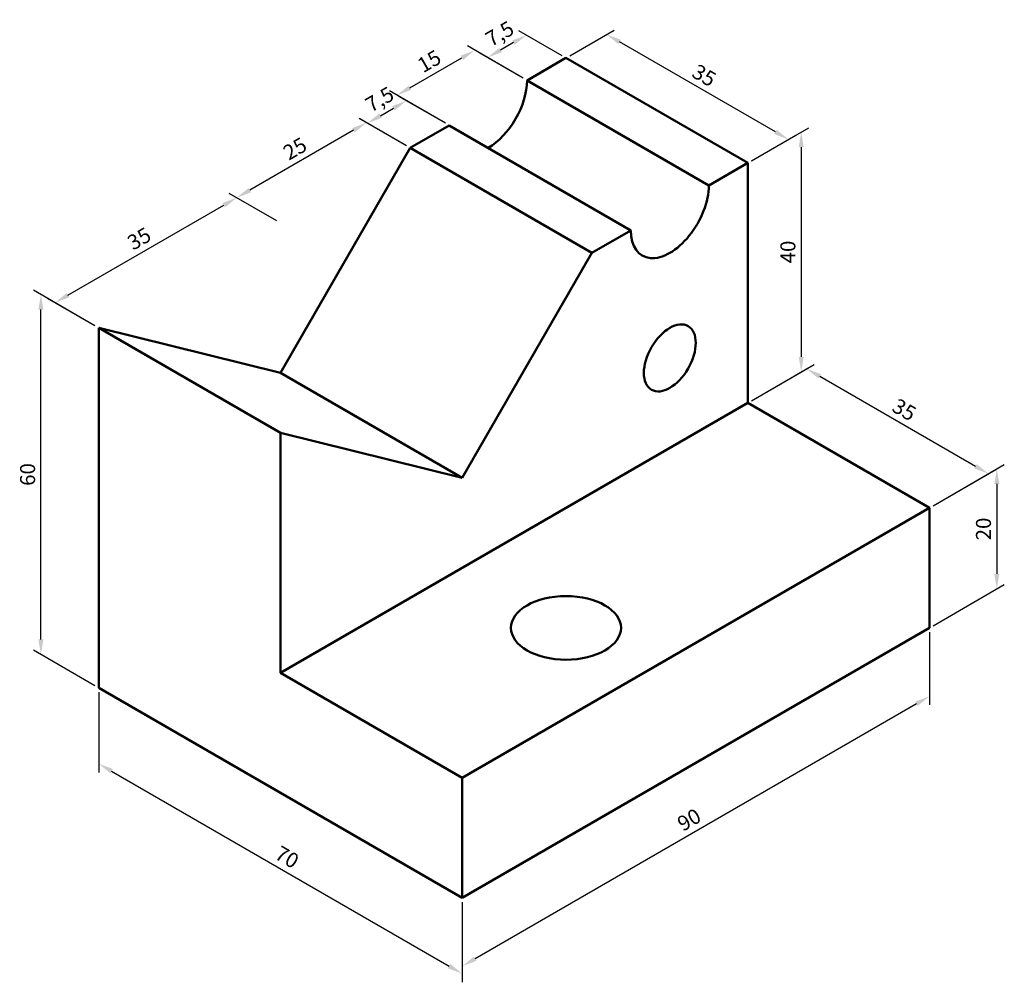
# Model space of a CAD drawing. Units: millimetres. Extents: x 1933 to 2097, y 2342 to 2503.
import ezdxf

# ---------------------------------------------------------------- set-up
doc = ezdxf.new("R2010")
doc.units = ezdxf.units.MM
doc.layers.add('M-DIMS', color=2, linetype='Continuous', lineweight=25)
doc.layers.add('M-OUTL', color=7, linetype='Continuous', lineweight=50)
doc.styles.get("Standard").update_dxf_attribs({"font": 'arial.ttf'})
doc.dimstyles.new('ISO-25', dxfattribs={"dimtxt": 2.5, "dimasz": 2.5, "dimexe": 1.25, "dimexo": 0.625, "dimtad": 1, "dimtxsty": 'Standard', "dimcen": 2.5, "dimadec": 0, "dimazin": 0, "dimtfac": 1, "dimtmove": 0, "dimatfit": 3, "dimfxl": 1, "dimarcsym": 0})

# ---------------------------------------------------------------- blocks, each defined once
blk = doc.blocks.new('*D1')
at = {"layer": 'Defpoints', "color": 0, "transparency": 16777216}
for p in [(2084.43, 2401.38), (2006.49, 2356.38), (2006.49, 2344.97)]:
    blk.add_point(p, dxfattribs=at)
at = {"layer": 'M-DIMS', "color": 0, "lineweight": -2, "transparency": 16777216}
for p, q in [((2084.43, 2400.65), (2084.43, 2388.53)), ((2082.27, 2388.72), (2008.66, 2346.22)), ((2006.49, 2355.65), (2006.49, 2343.53))]:
    blk.add_line(p, q, dxfattribs=at)
at = {"layer": 'M-DIMS', "color": 0, "transparency": 16777216}
for points in [[(2082.06, 2389.08), (2082.48, 2388.36), (2084.43, 2389.97)], [(2008.45, 2346.58), (2008.86, 2345.86), (2006.49, 2344.97)]]:
    blk.add_solid(points, dxfattribs=at)
at = {"layer": 'M-DIMS', "color": 0, "transparency": 16777216, "insert": (2044.51, 2369.12), "char_height": 2.5, "attachment_point": 5, "rotation": 30}
blk.add_mtext('90', dxfattribs=at)
blk = doc.blocks.new('*D2')
at = {"layer": 'Defpoints', "color": 0, "transparency": 16777216}
for p in [(2084.43, 2421.38), (2095.67, 2407.86), (2084.43, 2401.38)]:
    blk.add_point(p, dxfattribs=at)
at = {"layer": 'M-DIMS', "color": 0, "lineweight": -2, "transparency": 16777216}
for p, q in [((2085.06, 2421.74), (2096.92, 2428.59)), ((2095.67, 2425.36), (2095.67, 2410.36)), ((2085.06, 2401.74), (2096.92, 2408.59))]:
    blk.add_line(p, q, dxfattribs=at)
at = {"layer": 'M-DIMS', "color": 0, "transparency": 16777216}
for points in [[(2095.26, 2425.36), (2096.09, 2425.36), (2095.67, 2427.86)], [(2095.26, 2410.36), (2096.09, 2410.36), (2095.67, 2407.86)]]:
    blk.add_solid(points, dxfattribs=at)
at = {"layer": 'M-DIMS', "color": 0, "transparency": 16777216, "insert": (2093.77, 2417.86), "char_height": 2.5, "attachment_point": 5, "rotation": 90}
blk.add_mtext('20', dxfattribs=at)
blk = doc.blocks.new('*D3')
at = {"layer": 'Defpoints', "color": 0, "transparency": 16777216}
for p in [(2054.12, 2438.88), (2094.28, 2427.06), (2084.43, 2421.38)]:
    blk.add_point(p, dxfattribs=at)
at = {"layer": 'M-DIMS', "color": 0, "lineweight": -2, "transparency": 16777216}
for p, q in [((2054.75, 2439.24), (2065.22, 2445.28)), ((2066.14, 2443.31), (2092.12, 2428.31)), ((2085.06, 2421.74), (2095.53, 2427.78))]:
    blk.add_line(p, q, dxfattribs=at)
at = {"layer": 'M-DIMS', "color": 0, "transparency": 16777216}
for points in [[(2066.34, 2443.67), (2065.93, 2442.95), (2063.97, 2444.56)], [(2092.32, 2428.67), (2091.91, 2427.95), (2094.28, 2427.06)]]:
    blk.add_solid(points, dxfattribs=at)
at = {"layer": 'M-DIMS', "color": 0, "transparency": 16777216, "insert": (2080.08, 2437.46), "char_height": 2.5, "attachment_point": 5, "rotation": 330}
blk.add_mtext('35', dxfattribs=at)
blk = doc.blocks.new('*D4')
at = {"layer": 'Defpoints', "color": 0, "transparency": 16777216}
for p in [(2054.12, 2478.88), (2063.05, 2444.03), (2054.12, 2438.88)]:
    blk.add_point(p, dxfattribs=at)
at = {"layer": 'M-DIMS', "color": 0, "lineweight": -2, "transparency": 16777216}
for p, q in [((2054.75, 2479.24), (2064.3, 2484.75)), ((2063.05, 2481.53), (2063.05, 2446.53)), ((2054.75, 2439.24), (2064.3, 2444.75))]:
    blk.add_line(p, q, dxfattribs=at)
at = {"layer": 'M-DIMS', "color": 0, "transparency": 16777216}
for points in [[(2062.63, 2481.53), (2063.47, 2481.53), (2063.05, 2484.03)], [(2062.63, 2446.53), (2063.47, 2446.53), (2063.05, 2444.03)]]:
    blk.add_solid(points, dxfattribs=at)
at = {"layer": 'M-DIMS', "color": 0, "transparency": 16777216, "insert": (2061.15, 2464.03), "char_height": 2.5, "attachment_point": 5, "rotation": 90}
blk.add_mtext('40', dxfattribs=at)
blk = doc.blocks.new('*D5')
at = {"layer": 'Defpoints', "color": 0, "transparency": 16777216}
for p in [(2030.6, 2500.29), (2023.81, 2496.38), (2054.12, 2478.88)]:
    blk.add_point(p, dxfattribs=at)
at = {"layer": 'M-DIMS', "color": 0, "lineweight": -2, "transparency": 16777216}
for p, q in [((2024.44, 2496.74), (2031.85, 2501.02)), ((2058.75, 2484.04), (2032.76, 2499.04)), ((2054.75, 2479.24), (2062.16, 2483.52))]:
    blk.add_line(p, q, dxfattribs=at)
at = {"layer": 'M-DIMS', "color": 0, "transparency": 16777216}
for points in [[(2032.97, 2499.41), (2032.56, 2498.68), (2030.6, 2500.29)], [(2058.95, 2484.41), (2058.54, 2483.68), (2060.91, 2482.79)]]:
    blk.add_solid(points, dxfattribs=at)
at = {"layer": 'M-DIMS', "color": 0, "transparency": 16777216, "insert": (2046.71, 2493.19), "char_height": 2.5, "attachment_point": 5, "rotation": 330}
blk.add_mtext('35', dxfattribs=at)
blk = doc.blocks.new('*D6')
at = {"layer": 'Defpoints', "color": 0, "transparency": 16777216}
for p in [(2010.72, 2496.43), (2023.81, 2496.38), (2017.32, 2492.63)]:
    blk.add_point(p, dxfattribs=at)
at = {"layer": 'M-DIMS', "color": 0, "lineweight": -2, "transparency": 16777216}
for p, q in [((2023.19, 2496.74), (2015.97, 2500.9)), ((2015.05, 2498.93), (2012.89, 2497.68)), ((2016.69, 2492.99), (2009.47, 2497.15))]:
    blk.add_line(p, q, dxfattribs=at)
at = {"layer": 'M-DIMS', "color": 0, "transparency": 16777216}
for points in [[(2014.84, 2499.29), (2015.26, 2498.57), (2017.22, 2500.18)], [(2012.68, 2498.04), (2013.1, 2497.32), (2010.72, 2496.43)]]:
    blk.add_solid(points, dxfattribs=at)
at = {"layer": 'M-DIMS', "color": 0, "transparency": 16777216, "insert": (2012.91, 2500.15), "char_height": 2.5, "attachment_point": 5, "rotation": 30}
blk.add_mtext('7,5', dxfattribs=at)
blk = doc.blocks.new('*D7')
at = {"layer": 'Defpoints', "color": 0, "transparency": 16777216}
for p in [(2008.61, 2497.65), (2017.32, 2492.63), (2004.33, 2485.13)]:
    blk.add_point(p, dxfattribs=at)
at = {"layer": 'M-DIMS', "color": 0, "lineweight": -2, "transparency": 16777216}
for p, q in [((2016.69, 2492.99), (2007.36, 2498.37)), ((1997.79, 2491.4), (2006.45, 2496.4)), ((2003.7, 2485.49), (1994.37, 2490.87))]:
    blk.add_line(p, q, dxfattribs=at)
at = {"layer": 'M-DIMS', "color": 0, "transparency": 16777216}
for points in [[(2006.24, 2496.76), (2006.65, 2496.04), (2008.61, 2497.65)], [(1997.58, 2491.76), (1997.99, 2491.04), (1995.62, 2490.15)]]:
    blk.add_solid(points, dxfattribs=at)
at = {"layer": 'M-DIMS', "color": 0, "transparency": 16777216, "insert": (2001.17, 2495.55), "char_height": 2.5, "attachment_point": 5, "rotation": 30}
blk.add_mtext('15', dxfattribs=at)
blk = doc.blocks.new('*D8')
at = {"layer": 'Defpoints', "color": 0, "transparency": 16777216}
for p in [(1997.2, 2489.24), (2004.33, 2485.13), (1997.83, 2481.38)]:
    blk.add_point(p, dxfattribs=at)
at = {"layer": 'M-DIMS', "color": 0, "lineweight": -2, "transparency": 16777216}
for p, q in [((2003.7, 2485.49), (1995.95, 2489.96)), ((1992.87, 2486.74), (1995.03, 2487.99)), ((1997.21, 2481.74), (1989.45, 2486.21))]:
    blk.add_line(p, q, dxfattribs=at)
at = {"layer": 'M-DIMS', "color": 0, "transparency": 16777216}
for points in [[(1994.83, 2488.35), (1995.24, 2487.63), (1997.2, 2489.24)], [(1992.66, 2487.1), (1993.08, 2486.38), (1990.7, 2485.49)]]:
    blk.add_solid(points, dxfattribs=at)
at = {"layer": 'M-DIMS', "color": 0, "transparency": 16777216, "insert": (1992.89, 2489.2), "char_height": 2.5, "attachment_point": 5, "rotation": 30}
blk.add_mtext('7,5', dxfattribs=at)
blk = doc.blocks.new('*D9')
at = {"layer": 'Defpoints', "color": 0, "transparency": 16777216}
for p in [(1997.83, 2481.38), (1968.9, 2473.08), (1976.18, 2468.88)]:
    blk.add_point(p, dxfattribs=at)
at = {"layer": 'M-DIMS', "color": 0, "lineweight": -2, "transparency": 16777216}
for p, q in [((1997.21, 2481.74), (1989.3, 2486.3)), ((1988.39, 2484.33), (1971.07, 2474.33)), ((1975.56, 2469.24), (1967.65, 2473.8))]:
    blk.add_line(p, q, dxfattribs=at)
at = {"layer": 'M-DIMS', "color": 0, "transparency": 16777216}
for points in [[(1988.18, 2484.69), (1988.59, 2483.97), (1990.55, 2485.58)], [(1970.86, 2474.69), (1971.27, 2473.97), (1968.9, 2473.08)]]:
    blk.add_solid(points, dxfattribs=at)
at = {"layer": 'M-DIMS', "color": 0, "transparency": 16777216, "insert": (1978.77, 2480.98), "char_height": 2.5, "attachment_point": 5, "rotation": 30}
blk.add_mtext('25', dxfattribs=at)
blk = doc.blocks.new('*D10')
at = {"layer": 'Defpoints', "color": 0, "transparency": 16777216}
for p in [(1968.9, 2473.08), (1976.18, 2468.88), (1945.87, 2451.38)]:
    blk.add_point(p, dxfattribs=at)
at = {"layer": 'M-DIMS', "color": 0, "lineweight": -2, "transparency": 16777216}
for p, q in [((1975.56, 2469.24), (1967.65, 2473.8)), ((1940.75, 2456.83), (1966.74, 2471.83)), ((1945.24, 2451.74), (1937.34, 2456.3))]:
    blk.add_line(p, q, dxfattribs=at)
at = {"layer": 'M-DIMS', "color": 0, "transparency": 16777216}
for points in [[(1966.53, 2472.19), (1966.94, 2471.47), (1968.9, 2473.08)], [(1940.55, 2457.19), (1940.96, 2456.47), (1938.59, 2455.58)]]:
    blk.add_solid(points, dxfattribs=at)
at = {"layer": 'M-DIMS', "color": 0, "transparency": 16777216, "insert": (1952.79, 2465.98), "char_height": 2.5, "attachment_point": 5, "rotation": 30}
blk.add_mtext('35', dxfattribs=at)
blk = doc.blocks.new('*D11')
at = {"layer": 'Defpoints', "color": 0, "transparency": 16777216}
for p in [(1936.24, 2456.94), (1945.87, 2451.38), (1945.87, 2391.38)]:
    blk.add_point(p, dxfattribs=at)
at = {"layer": 'M-DIMS', "color": 0, "lineweight": -2, "transparency": 16777216}
for p, q in [((1945.24, 2451.74), (1934.99, 2457.66)), ((1936.24, 2399.44), (1936.24, 2454.44)), ((1945.24, 2391.74), (1934.99, 2397.66))]:
    blk.add_line(p, q, dxfattribs=at)
at = {"layer": 'M-DIMS', "color": 0, "transparency": 16777216}
for points in [[(1935.82, 2454.44), (1936.66, 2454.44), (1936.24, 2456.94)], [(1935.82, 2399.44), (1936.66, 2399.44), (1936.24, 2396.94)]]:
    blk.add_solid(points, dxfattribs=at)
at = {"layer": 'M-DIMS', "color": 0, "transparency": 16777216, "insert": (1934.34, 2426.94), "char_height": 2.5, "attachment_point": 5, "rotation": 90}
blk.add_mtext('60', dxfattribs=at)
blk = doc.blocks.new('*D12')
at = {"layer": 'Defpoints', "color": 0, "transparency": 16777216}
for p in [(1945.87, 2391.38), (2006.49, 2356.38), (2006.49, 2343.74)]:
    blk.add_point(p, dxfattribs=at)
at = {"layer": 'M-DIMS', "color": 0, "lineweight": -2, "transparency": 16777216}
for p, q in [((1945.87, 2390.65), (1945.87, 2377.29)), ((1948.03, 2377.49), (2004.33, 2344.99)), ((2006.49, 2355.65), (2006.49, 2342.29))]:
    blk.add_line(p, q, dxfattribs=at)
at = {"layer": 'M-DIMS', "color": 0, "transparency": 16777216}
for points in [[(1948.24, 2377.85), (1947.83, 2377.13), (1945.87, 2378.74)], [(2004.53, 2345.35), (2004.12, 2344.63), (2006.49, 2343.74)]]:
    blk.add_solid(points, dxfattribs=at)
at = {"layer": 'M-DIMS', "color": 0, "transparency": 16777216, "insert": (1977.13, 2362.88), "char_height": 2.5, "attachment_point": 5, "rotation": 330}
blk.add_mtext('70', dxfattribs=at)

msp = doc.modelspace()

# ---------------------------------------------------------------- linework, layer by layer
at = {"layer": 'M-OUTL'}
for p, q in [((2023.812, 2496.376), (2017.317, 2492.626)), ((2054.123, 2478.876), (2023.812, 2496.376)), ((2017.317, 2492.626), (2047.628, 2475.126)), ((1997.831, 2481.376), (2004.326, 2485.126)), ((2004.326, 2485.126), (2034.637, 2467.626)), ((1976.181, 2443.876), (1997.831, 2481.376)), ((2028.142, 2463.876), (1997.831, 2481.376)), ((2047.628, 2475.126), (2054.123, 2478.876)), ((2054.123, 2438.876), (2054.123, 2478.876)), ((2034.637, 2467.626), (2028.142, 2463.876)), ((2006.491, 2426.376), (2028.142, 2463.876)), ((1945.87, 2451.376), (1945.87, 2391.376)), ((1976.181, 2433.876), (1945.87, 2451.376)), ((1976.181, 2443.876), (1945.87, 2451.376)), ((2006.491, 2426.376), (1976.181, 2443.876)), ((1976.181, 2393.876), (2054.123, 2438.876)), ((2054.123, 2438.876), (2084.434, 2421.376)), ((1976.181, 2393.876), (1976.181, 2433.876)), ((2006.491, 2426.376), (1976.181, 2433.876)), ((2084.434, 2421.376), (2006.491, 2376.376)), ((2084.434, 2401.376), (2084.434, 2421.376)), ((2006.491, 2356.376), (2084.434, 2401.376)), ((2006.491, 2376.376), (1976.181, 2393.876)), ((1945.87, 2391.376), (2006.491, 2356.376)), ((2006.491, 2376.376), (2006.491, 2356.376))]:
    msp.add_line(p, q, dxfattribs=at)
for centre, start_param in [((2010.822, 2488.876), 7.0685835), ((2041.133, 2471.376), 5.4977871)]:
    msp.add_ellipse(centre, major_axis=(-4.593, -7.955), ratio=0.5773503, start_param=start_param, end_param=8.6393798, dxfattribs=at)
for centre, major_axis in [((2041.133, 2446.376), (-3.062, -5.303)), ((2023.812, 2401.376), (-9.186, 0))]:
    msp.add_ellipse(centre, major_axis=major_axis, ratio=0.5773503, dxfattribs=at)

# ---------------------------------------------------------------- dimensions: what is measured, and where the dimension line sits
at = {"layer": 'M-DIMS'}
for p1, p2, distance, picture, middle in [((2023.812, 2496.376), (2017.317, 2492.626), -6.594, '*D6', (2012.91, 2500.146)), ((2054.123, 2478.876), (2023.812, 2496.376), -6.788, '*D5', (2046.706, 2493.192)), ((2004.326, 2485.126), (2017.317, 2492.626), 8.706, '*D7', (2001.165, 2495.549)), ((1997.831, 2481.376), (2004.326, 2485.126), 7.127, '*D8', (1992.891, 2489.204)), ((1997.831, 2481.376), (1976.181, 2468.876), -7.28, '*D9', (1978.775, 2480.976)), ((2054.123, 2478.876), (2054.123, 2438.876), 8.926, '*D4', (2061.148, 2464.03)), ((1945.87, 2451.376), (1976.181, 2468.876), 7.28, '*D10', (1952.794, 2465.977)), ((1945.87, 2391.376), (1945.87, 2451.376), 9.631, '*D11', (1934.338, 2426.936)), ((2054.123, 2438.876), (2084.434, 2421.376), 9.848, '*D3', (2080.077, 2437.459)), ((2084.434, 2421.376), (2084.434, 2401.376), 11.238, '*D2', (2093.77, 2417.864)), ((2084.434, 2401.376), (2006.491, 2356.376), 9.876, '*D1', (2044.512, 2369.119)), ((1945.87, 2391.376), (2006.491, 2356.376), -10.945, '*D12', (1977.131, 2362.885))]:
    dim = msp.add_aligned_dim(p1=p1, p2=p2, distance=distance, dimstyle='ISO-25', override={"dimclrd": 0, "dimclre": 0, "dimclrt": 0}, dxfattribs=at)
    dim.commit()
    dim.dimension.update_dxf_attribs({"geometry": picture, "text_midpoint": middle})

doc.saveas('drawing.dxf')
